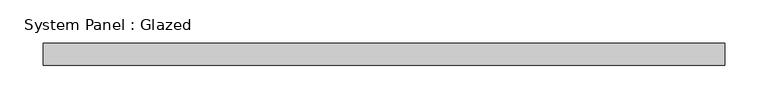
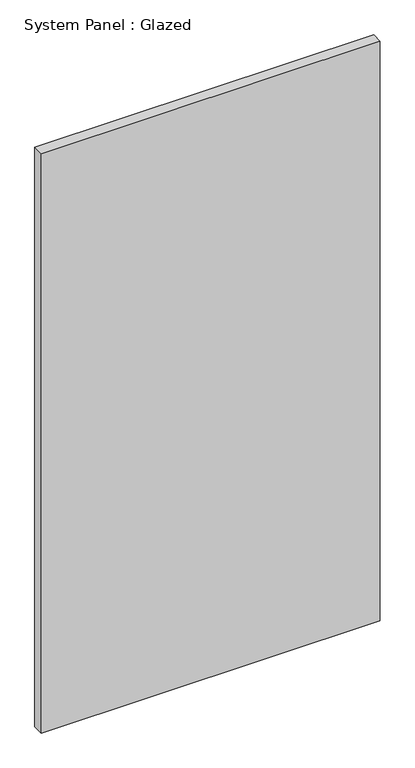
"""IFC4 building model written with IfcOpenShell, lengths in millimetres: plate geometry, System Panel : Glazed."""

from ifc_helpers import new_model, si_unit, origin, origin_with_axes, place, context, project, spatial, polyline, outline, extrude, source, transform, mapped, element, save


def system_panel_glazed_b0c11670(model_context):
    return source(origin(), model_context, "Body", "SweptSolid", [
        extrude(outline(polyline([(393.7, 19.05), (-393.7, 19.05), (-393.7, 44.45), (393.7, 44.45), (393.7, 19.05)])), origin_with_axes(), (0.0, 0.0, 1.0), 1422.4),
    ])


if __name__ == "__main__":
    model = new_model("IFC4")
    model_context = context("Model", 3, world=origin())
    ifc_project = project(units=[si_unit("LENGTHUNIT", "METRE", prefix="MILLI")], contexts=[model_context])
    site = spatial("IfcSite", under=ifc_project)
    building = spatial("IfcBuilding", under=site)
    placement = place(None, origin())
    system_panel_glazed_shape = system_panel_glazed_b0c11670(model_context)
    element("IfcPlate", 1, ObjectType="System Panel : Glazed", at=placement, inside=building, context=model_context, shape_type="MappedRepresentation", body=[
        mapped(system_panel_glazed_shape, transform((0.0, 0.0, 0.0), x_axis=(1.0, 0.0, 0.0), y_axis=(0.0, 1.0, 0.0), z_axis=(0.0, 0.0, 1.0))),
    ])
    save(model, "model.ifc")

# Revit data of these elements
# Type "System Panel : Glazed"
#   Construction Type Id = "GSP4R"
#   Analytic Construction = "1/8 in Pilkington single glazing"
#   Visual Light Transmittance = 0.9
#   Solar Heat Gain Coefficient = 0.86
#   Heat Transfer Coefficient (U) = 1.18115 BTU/(h·ft²·°F)
#   Define Thermal Properties by = 1
# Element 1 (IfcPlate, "System Panel : Glazed")
#   Materials on its faces: "Glass"
# Materials
#   "Glass": class "Glass", colour RGB 0 128 192, transparency 0.75, Description = "Soda Lime Glass", Cost = 0
